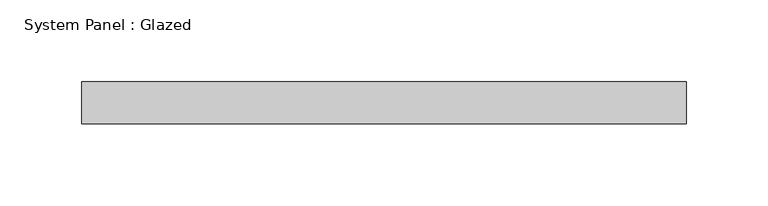
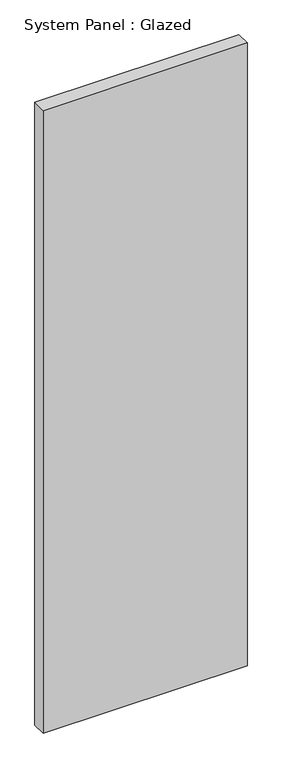
"""IFC4 building model written with IfcOpenShell, lengths in millimetres: plate geometry, System Panel : Glazed."""

from ifc_helpers import new_model, si_unit, origin, origin_with_axes, place, context, project, spatial, polyline, outline, extrude, source, transform, mapped, element, save


def system_panel_glazed_f9e68b79(model_context):
    return source(origin(), model_context, "Body", "SweptSolid", [
        extrude(outline(polyline([(184.15, 19.05), (-184.15, 19.05), (-184.15, 44.45), (184.15, 44.45), (184.15, 19.05)])), origin_with_axes(), (0.0, 0.0, 1.0), 1188.425758),
    ])


if __name__ == "__main__":
    model = new_model("IFC4")
    model_context = context("Model", 3, world=origin())
    ifc_project = project(units=[si_unit("LENGTHUNIT", "METRE", prefix="MILLI")], contexts=[model_context])
    site = spatial("IfcSite", under=ifc_project)
    building = spatial("IfcBuilding", under=site)
    placement = place(None, origin())
    system_panel_glazed_shape = system_panel_glazed_f9e68b79(model_context)
    element("IfcPlate", 1, ObjectType="System Panel : Glazed", at=placement, inside=building, context=model_context, shape_type="MappedRepresentation", body=[
        mapped(system_panel_glazed_shape, transform((0.0, 0.0, 0.0), x_axis=(1.0, 0.0, 0.0), y_axis=(0.0, 1.0, 0.0), z_axis=(0.0, 0.0, 1.0))),
    ])
    save(model, "model.ifc")

# Revit data of these elements
# Type "System Panel : Glazed"
#   Construction Type Id = "GSP4R"
#   Analytic Construction = "1/8 in Pilkington single glazing"
#   Visual Light Transmittance = 0.9
#   Solar Heat Gain Coefficient = 0.86
#   Heat Transfer Coefficient (U) = 1.18115 BTU/(h·ft²·°F)
#   Define Thermal Properties by = 1
# Element 1 (IfcPlate, "System Panel : Glazed")
#   Materials on its faces: "Glass"
# Materials
#   "Glass": class "Glass", colour RGB 0 128 192, transparency 0.75, Description = "Soda Lime Glass", Cost = 0
